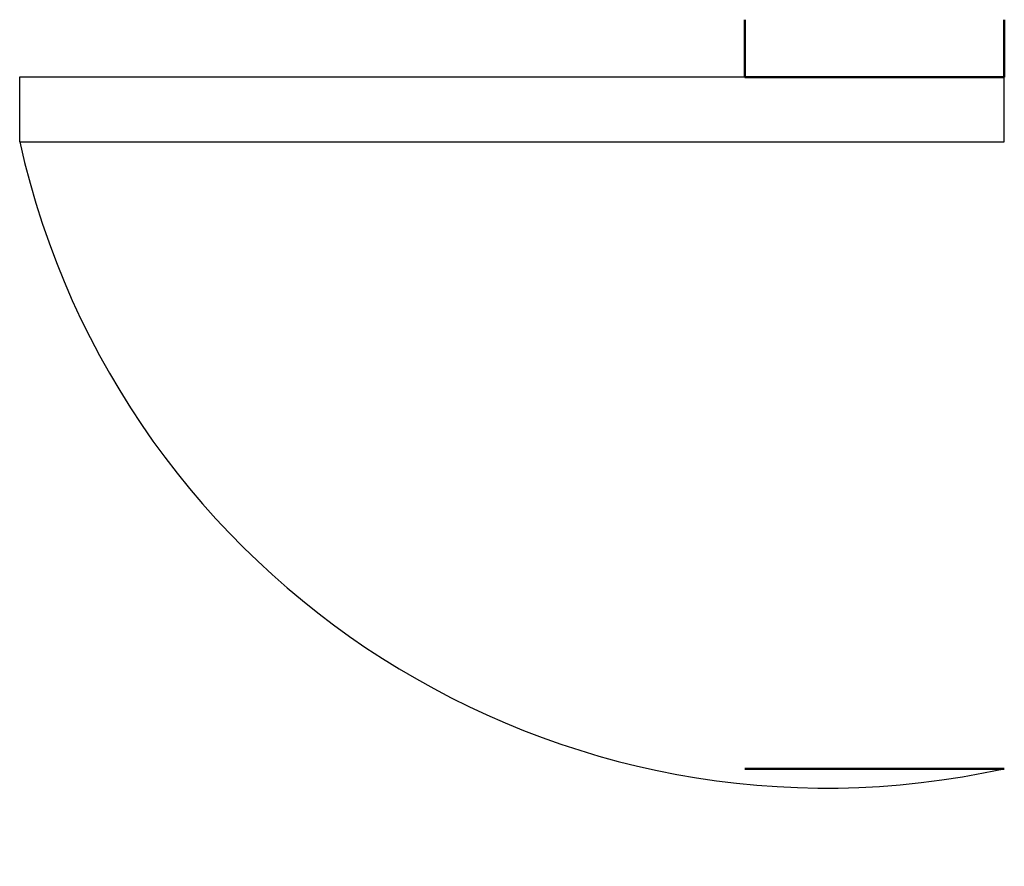
# Model space of a CAD drawing. Units: inches. Extents: x 2050 to 6806, y 2092 to 5743.
# Tile 8 of 8: x 6772 to 6806, y 5713 to 5743. Entities that reach past the tile are written whole.
import ezdxf

# ---------------------------------------------------------------- set-up
doc = ezdxf.new("R2010")
doc.units = ezdxf.units.IN
doc.layers.add('A-DOOR', color=2, linetype='Continuous', lineweight=25)
doc.layers.add('A-WALL', color=7, linetype='Continuous', lineweight=50)

# ---------------------------------------------------------------- blocks, each defined once
blk = doc.blocks.new('DOOR-700')
blk.add_lwpolyline([(34.147, 24.67), (0, 24.67), (0, 22.418), (34.147, 22.418)], close=True)
blk.add_arc((27.994, 28.691), 28.688, 192.6316, 282.383)

msp = doc.modelspace()

# ---------------------------------------------------------------- linework, layer by layer
at = {"layer": 'A-WALL'}
for p, q in [((6797.343, 5740.673), (6797.343, 5742.663)), ((6806.343, 5740.673), (6806.343, 5742.663)), ((6797.343, 5740.673), (6806.343, 5740.673)), ((6797.343, 5716.673), (6806.343, 5716.673))]:
    msp.add_line(p, q, dxfattribs=at)

# ---------------------------------------------------------------- block references
at = {"layer": 'A-DOOR'}
msp.add_blockref('DOOR-700', (6772.196, 5716.003), dxfattribs=at)

doc.saveas('drawing.dxf')
